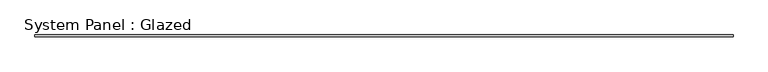
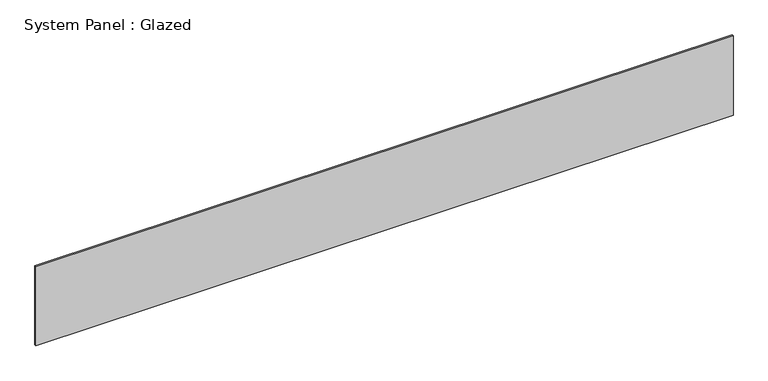
"""IFC4 building model written with IfcOpenShell, lengths in millimetres: plate geometry, System Panel : Glazed."""

from ifc_helpers import new_model, si_unit, origin, origin_with_axes, place, context, project, spatial, polyline, outline, extrude, source, transform, mapped, element, save


def system_panel_glazed_decb64e8(model_context):
    return source(origin(), model_context, "Body", "SweptSolid", [
        extrude(outline(polyline([(5080.0, 19.05), (-5080.0, 19.05), (-5080.0, 44.45), (5080.0, 44.45), (5080.0, 19.05)])), origin_with_axes(), (0.0, 0.0, 1.0), 1219.2),
    ])


if __name__ == "__main__":
    model = new_model("IFC4")
    model_context = context("Model", 3, world=origin())
    ifc_project = project(units=[si_unit("LENGTHUNIT", "METRE", prefix="MILLI")], contexts=[model_context])
    site = spatial("IfcSite", under=ifc_project)
    building = spatial("IfcBuilding", under=site)
    placement = place(None, origin())
    system_panel_glazed_shape = system_panel_glazed_decb64e8(model_context)
    element("IfcPlate", 1, ObjectType="System Panel : Glazed", at=placement, inside=building, context=model_context, shape_type="MappedRepresentation", body=[
        mapped(system_panel_glazed_shape, transform((0.0, 0.0, 0.0), x_axis=(1.0, 0.0, 0.0), y_axis=(0.0, 1.0, 0.0), z_axis=(0.0, 0.0, 1.0))),
    ])
    save(model, "model.ifc")

# Revit data of these elements
# Type "System Panel : Glazed"
#   Construction Type Id = "GSP4R"
#   Analytic Construction = "1/8 in Pilkington single glazing"
#   Visual Light Transmittance = 0.9
#   Solar Heat Gain Coefficient = 0.86
#   Heat Transfer Coefficient (U) = 1.18115 BTU/(h·ft²·°F)
# Element 1 (IfcPlate, "System Panel : Glazed")
#   Materials on its faces: "Glass"
# Materials
#   "Glass": class "Glass", colour RGB 0 128 192, transparency 0.75, Description = "Soda Lime Glass", Cost = 0
